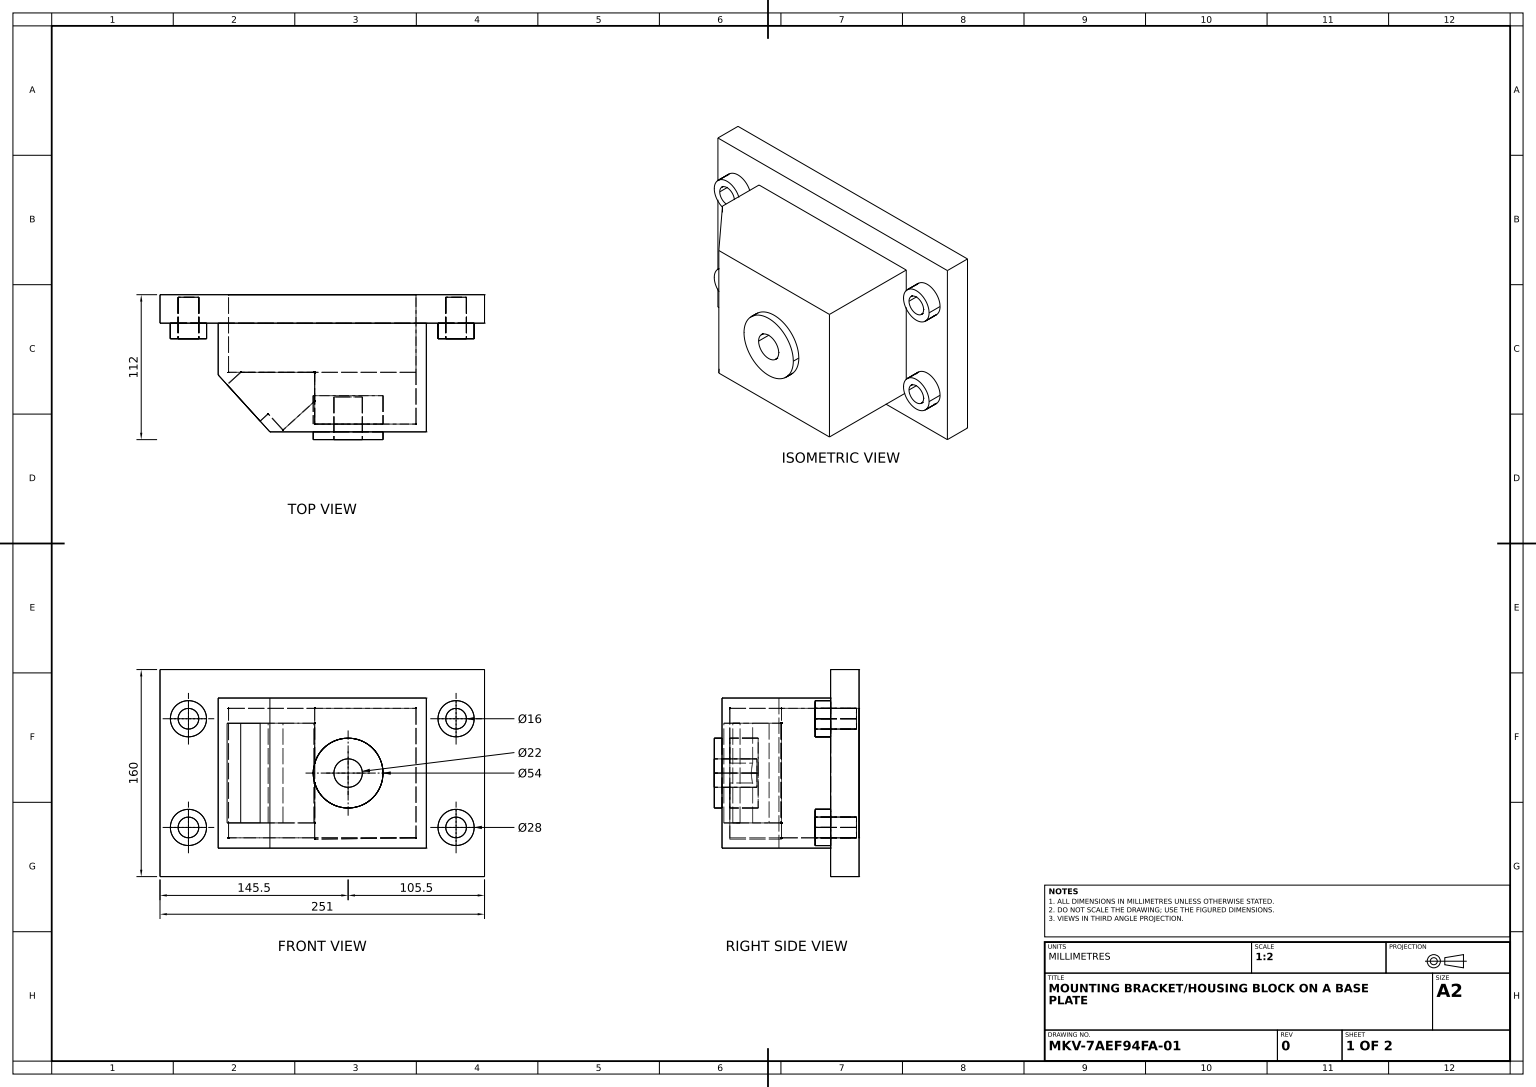
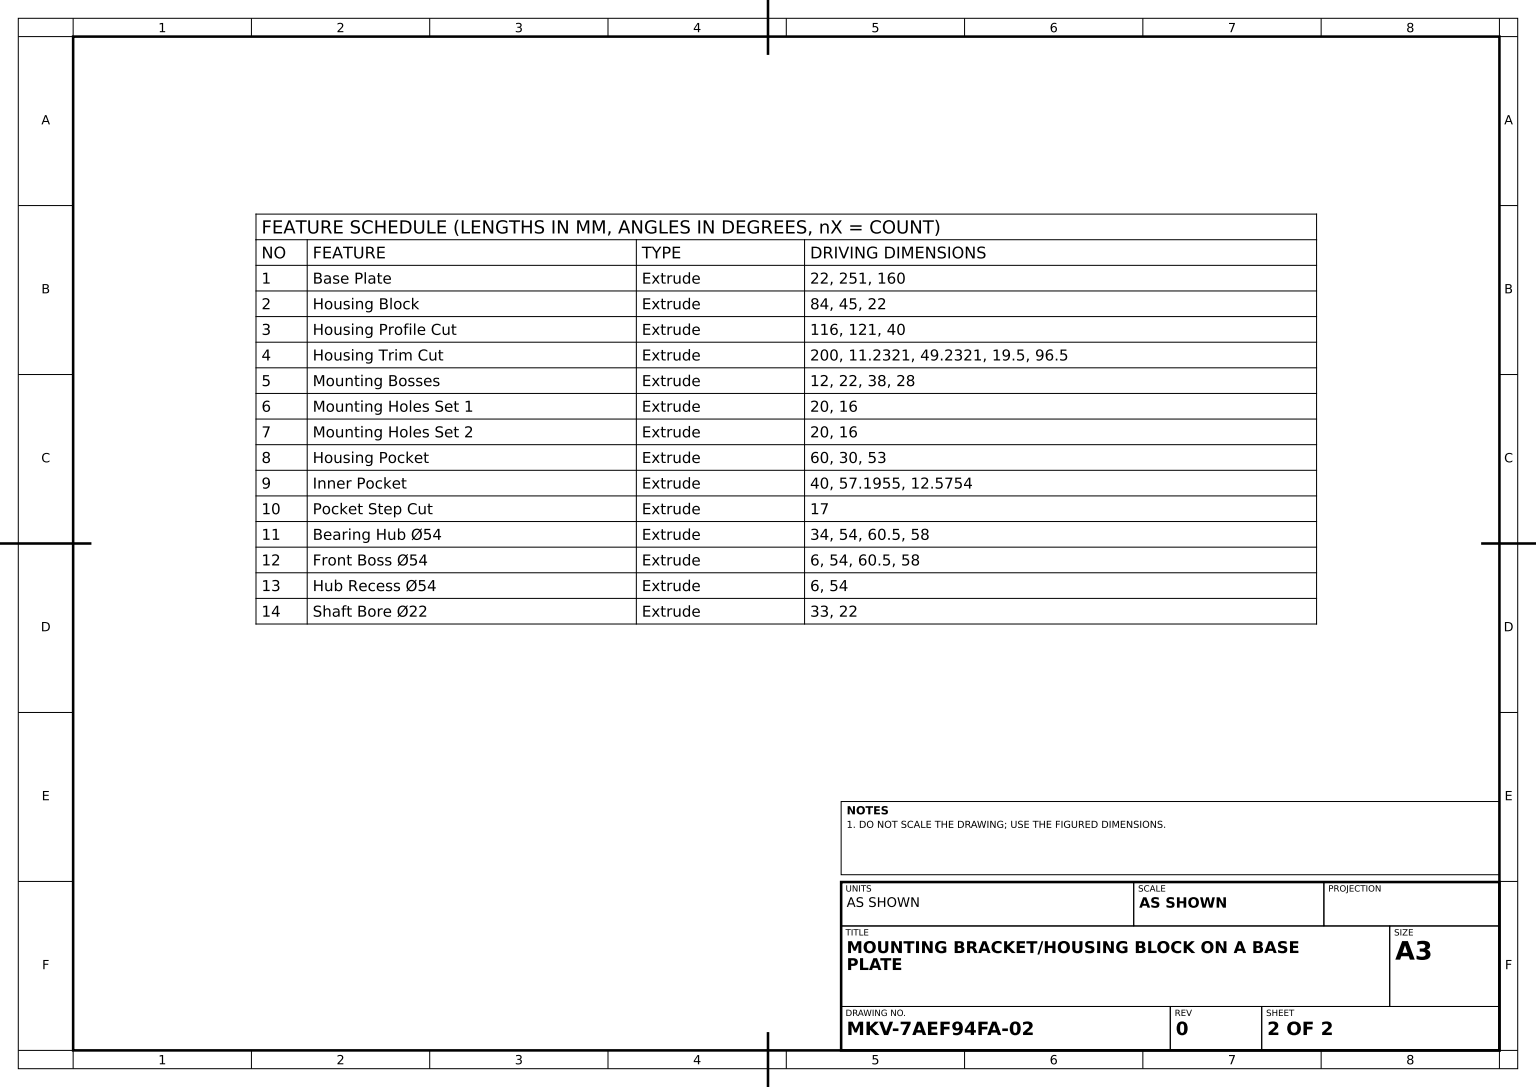
from build123d import *

# Parameters (mm, degrees)
BASE_PLATE_SKETCH_W           = 251
BASE_PLATE_SKETCH_H           = 160
BASE_PLATE_DEPTH              = 22
HOUSING_BLOCK_SKETCH_W        = 161
HOUSING_BLOCK_SKETCH_H        = 116
HOUSING_BLOCK_DEPTH           = 84
HOUSING_PROFILE_CUT_DEPTH     = 116
HOUSING_TRIM_CUT_SKETCH_W     = 38
HOUSING_TRIM_CUT_SKETCH_H     = 77
HOUSING_TRIM_CUT_DEPTH        = 200
MOUNTING_BOSSES_SKETCH_R      = 14
MOUNTING_BOSSES_DEPTH         = 12
MOUNTING_HOLES_SET_1_SKETCH_R = 8
MOUNTING_HOLES_SET_1_DEPTH    = 20
MOUNTING_HOLES_SET_2_SKETCH_R = 8
MOUNTING_HOLES_SET_2_DEPTH    = 20
HOUSING_POCKET_SKETCH_W       = 145
HOUSING_POCKET_SKETCH_H       = 100
HOUSING_POCKET_DEPTH          = 60
INNER_POCKET_DEPTH            = 40
POCKET_STEP_CUT_SKETCH_W      = 47.620155069
POCKET_STEP_CUT_SKETCH_H      = 77
POCKET_STEP_CUT_DEPTH         = 17
BEARING_HUB_54_SKETCH_R       = 27
BEARING_HUB_54_DEPTH          = 34
FRONT_START                   = 6
FRONT_BOSS_54_SKETCH_R        = 27
FRONT_BOSS_54_DEPTH           = 6
HUB_START                     = -6
HUB_RECESS_54_SKETCH_R        = 27
HUB_RECESS_54_DEPTH           = 6
SHAFT_BORE_22_SKETCH_R        = 11
SHAFT_BORE_22_DEPTH           = 33


with BuildPart() as part:
    # Base Plate Sketch → Base Plate (new body)
    with BuildSketch(Plane.XY):
        with Locations((125.5, 80)):
            Rectangle(BASE_PLATE_SKETCH_W, BASE_PLATE_SKETCH_H)
    extrude(amount=BASE_PLATE_DEPTH)

    # Housing Block Sketch → Housing Block (add)
    with BuildSketch(Plane.XY.offset(22)):
        with Locations((125.5, 80)):
            Rectangle(HOUSING_BLOCK_SKETCH_W, HOUSING_BLOCK_SKETCH_H)
    extrude(amount=HOUSING_BLOCK_DEPTH)

    # Housing Profile Cut Sketch → Housing Profile Cut (cut)
    with BuildSketch(Plane.XZ.offset(-22)):
        Polygon((85, 106), (45, 62), (45, 106), align=None)
    extrude(amount=-HOUSING_PROFILE_CUT_DEPTH, mode=Mode.SUBTRACT)

    # Housing Trim Cut Sketch → Housing Trim Cut (cut)
    with BuildSketch(Plane(origin=(-6.221719457, 0, 5.656108597), x_dir=(0.6726727939963125, 0, 0.7399400733959438), z_dir=(-0.7399400733959438, 0, 0.6726727939963125))):
        with Locations((105.378697775, 80)):
            Rectangle(HOUSING_TRIM_CUT_SKETCH_W, HOUSING_TRIM_CUT_SKETCH_H)
    extrude(amount=-HOUSING_TRIM_CUT_DEPTH, mode=Mode.SUBTRACT)

    # Mounting Bosses Sketch → Mounting Bosses (add)
    with BuildSketch(Plane.XY.offset(22)):
        with Locations((229, 122)):
            Circle(MOUNTING_BOSSES_SKETCH_R)
        with Locations((229, 38)):
            Circle(MOUNTING_BOSSES_SKETCH_R)
        with Locations((22, 38)):
            Circle(MOUNTING_BOSSES_SKETCH_R)
        with Locations((22, 122)):
            Circle(MOUNTING_BOSSES_SKETCH_R)
    extrude(amount=MOUNTING_BOSSES_DEPTH)

    # Mounting Holes Set 1 Sketch → Mounting Holes Set 1 (cut)
    with BuildSketch(Plane.XY.offset(22)):
        with Locations((22, 122)):
            Circle(MOUNTING_HOLES_SET_1_SKETCH_R)
        with Locations((22, 38)):
            Circle(MOUNTING_HOLES_SET_1_SKETCH_R)
        with Locations((229, 38)):
            Circle(MOUNTING_HOLES_SET_1_SKETCH_R)
        with Locations((229, 122)):
            Circle(MOUNTING_HOLES_SET_1_SKETCH_R)
    extrude(amount=-MOUNTING_HOLES_SET_1_DEPTH, mode=Mode.SUBTRACT)

    # Mounting Holes Set 2 Sketch → Mounting Holes Set 2 (cut)
    with BuildSketch(Plane.XY.offset(34)):
        with Locations((229, 122)):
            Circle(MOUNTING_HOLES_SET_2_SKETCH_R)
        with Locations((229, 38)):
            Circle(MOUNTING_HOLES_SET_2_SKETCH_R)
        with Locations((22, 38)):
            Circle(MOUNTING_HOLES_SET_2_SKETCH_R)
        with Locations((22, 122)):
            Circle(MOUNTING_HOLES_SET_2_SKETCH_R)
    extrude(amount=-MOUNTING_HOLES_SET_2_DEPTH, mode=Mode.SUBTRACT)

    # Housing Pocket Sketch → Housing Pocket (cut)
    with BuildSketch(Plane(origin=(0, 0, 0), x_dir=(-1, 0, 0), z_dir=(0, 0, -1))):
        with Locations((-125.5, 80)):
            Rectangle(HOUSING_POCKET_SKETCH_W, HOUSING_POCKET_SKETCH_H)
    extrude(amount=-HOUSING_POCKET_DEPTH, mode=Mode.SUBTRACT)

    # Inner Pocket Sketch → Inner Pocket (cut)
    with BuildSketch(Plane(origin=(0, 0, 60), x_dir=(-1, 0, 0), z_dir=(0, 0, -1))):
        Polygon((-198, 130), (-119.606684276, 130), (-119.606684276, 28.92459706), (-198, 30), align=None)
    extrude(amount=-INNER_POCKET_DEPTH, mode=Mode.SUBTRACT)

    # Pocket Step Cut Sketch → Pocket Step Cut (cut)
    with BuildSketch(Plane(origin=(83.666166146, 0, 92.032782761), x_dir=(-0.7399400733959437, 0, 0.6726727939963125), z_dir=(-0.6726727939963125, 0, -0.7399400733959437))):
        with Locations((-23.810077535, 80)):
            Rectangle(POCKET_STEP_CUT_SKETCH_W, POCKET_STEP_CUT_SKETCH_H)
    extrude(amount=-POCKET_STEP_CUT_DEPTH, mode=Mode.SUBTRACT)

    # Bearing Hub Ø54 Sketch → Bearing Hub Ø54 (add)
    with BuildSketch(Plane.XY.offset(106)):
        with Locations((145.5, 80)):
            Circle(BEARING_HUB_54_SKETCH_R)
    extrude(amount=-BEARING_HUB_54_DEPTH)

    # Front Boss Ø54 Sketch → Front Boss Ø54 (add)
    with BuildSketch(Plane.XY.offset(106).offset(FRONT_START)):
        with Locations((145.5, 80)):
            Circle(FRONT_BOSS_54_SKETCH_R)
    extrude(amount=-FRONT_BOSS_54_DEPTH)

    # Hub Recess Ø54 Sketch → Hub Recess Ø54 (cut)
    with BuildSketch(Plane(origin=(0, 0, 72), x_dir=(-1, 0, 0), z_dir=(0, 0, -1)).offset(HUB_START)):
        with Locations(Location((-145.5, 80, 0), (0, 0, 16.461230985))):
            Circle(HUB_RECESS_54_SKETCH_R)
    extrude(amount=HUB_RECESS_54_DEPTH, mode=Mode.SUBTRACT)

    # Shaft Bore Ø22 Sketch → Shaft Bore Ø22 (cut)
    with BuildSketch(Plane.XY.offset(112)):
        with Locations((145.5, 80)):
            Circle(SHAFT_BORE_22_SKETCH_R)
    extrude(amount=-SHAFT_BORE_22_DEPTH, mode=Mode.SUBTRACT)


solid = part.part
